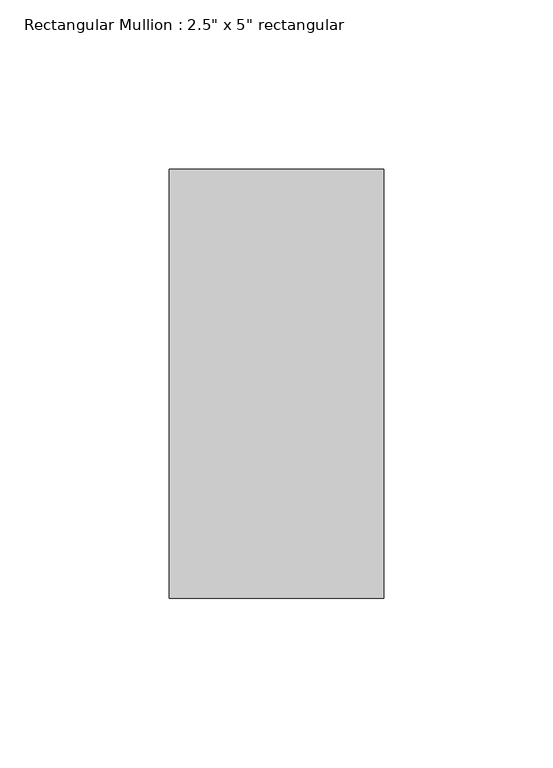
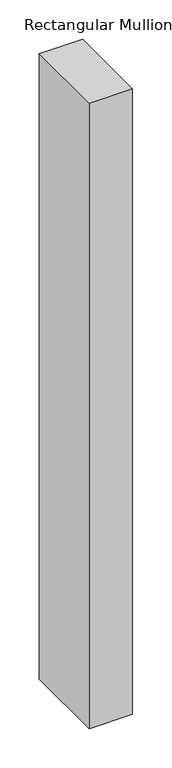
"""IFC4 building model written with IfcOpenShell, lengths in millimetres: member geometry."""

from ifc_helpers import new_model, si_unit, frame, origin, place, context, project, spatial, polyline, outline, extrude, source, transform, mapped, element, save


def member_0998ace5(model_context):
    return source(origin(), model_context, "Body", "SweptSolid", [
        extrude(outline(polyline([(31.75, 63.5), (31.75, -63.5), (-31.75, -63.5), (-31.75, 63.5), (31.75, 63.5)])), frame((0.0, 0.0, -971.5500001), z_axis=(0.0, 0.0, 1.0), x_axis=(1.0, 0.0, 0.0)), (0.0, 0.0, 1.0), 971.5500001),
    ])


if __name__ == "__main__":
    model = new_model("IFC4")
    model_context = context("Model", 3, world=origin())
    ifc_project = project(units=[si_unit("LENGTHUNIT", "METRE", prefix="MILLI")], contexts=[model_context])
    site = spatial("IfcSite", under=ifc_project)
    building = spatial("IfcBuilding", under=site)
    placement = place(None, origin())
    member_shape = member_0998ace5(model_context)
    element("IfcMember", 1, ObjectType="Rectangular Mullion : 2.5\" x 5\" rectangular", at=placement, inside=building, context=model_context, shape_type="MappedRepresentation", body=[
        mapped(member_shape, transform((0.0, 0.0, 0.0), x_axis=(1.0, 0.0, 0.0), y_axis=(0.0, 1.0, 0.0), z_axis=(0.0, 0.0, 1.0))),
    ])
    save(model, "model.ifc")

# Revit data of these elements
# Type "Rectangular Mullion : 2.5\" x 5\" rectangular"
#   built-in parameter 1007304 = 0.416667 (stored number, unit not read)
#   built-in parameter 1007301 = 0.104167 (stored number, unit not read)
#   built-in parameter 1007300 = 0.104167 (stored number, unit not read)
# Element 1 (IfcMember, "Rectangular Mullion : 2.5\" x 5\" rectangular")
#   Materials on its faces: "Aluminum"
# Materials
#   "Aluminum": class "Metal", colour RGB 247 247 247, transparency 0, Description = "Aluminum 6061", Cost = 0
